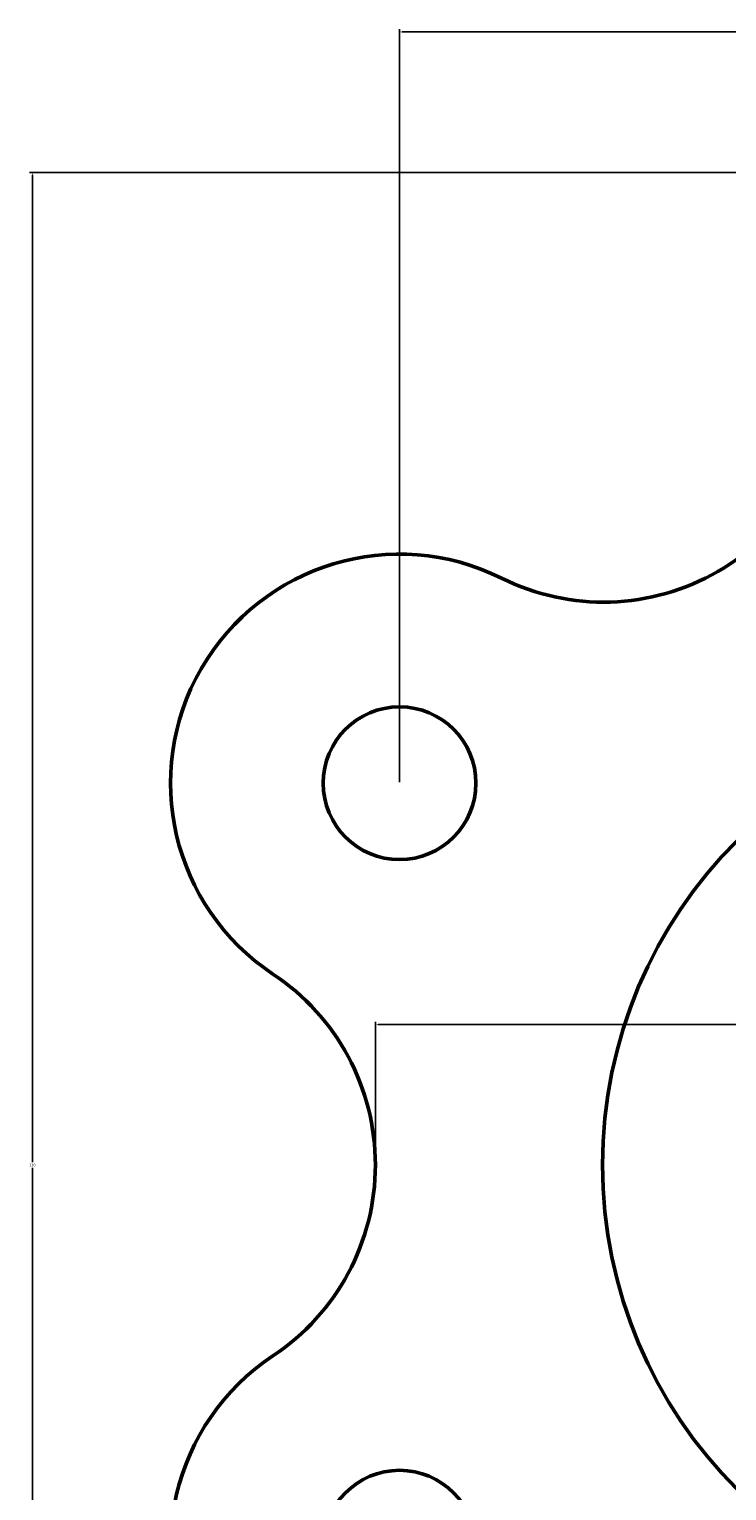
# Model space of a CAD drawing. Units: millimetres. Extents: x 2038 to 2173, y 1596 to 1745.
# Tile 2 of 4: x 2038 to 2084, y 1649 to 1745. Entities that reach past the tile are written whole.
import ezdxf

# ---------------------------------------------------------------- set-up
doc = ezdxf.new("R2010")
doc.units = ezdxf.units.MM
doc.layers.add('M-DIMS', color=2, linetype='Continuous', lineweight=18)
doc.layers.add('M-OUTL', color=7, linetype='Continuous', lineweight=50)
doc.styles.get("Standard").update_dxf_attribs({"font": 'arial.ttf'})
doc.dimstyles.get("Standard").update_dxf_attribs({"dimtxt": 0.18, "dimasz": 0.18, "dimexe": 0.18, "dimexo": 0.0625, "dimgap": 0.09, "dimtad": 0, "dimtih": 1, "dimtoh": 1, "dimdec": 4, "dimzin": 0, "dimdsep": 46, "dimtxsty": 'Standard', "dimcen": 0.09, "dimadec": 0, "dimazin": 0, "dimtfac": 1, "dimtdec": 4, "dimtofl": 0, "dimtmove": 0, "dimatfit": 3, "dimfxl": 1, "dimtolj": 1, "dimtzin": 0, "dimarcsym": 0})

# ---------------------------------------------------------------- blocks, each defined once
blk = doc.blocks.new('*U1')
blk.add_arc((-4.146, 7.965), 15, 243.55731, 356.44269)
blk = doc.blocks.new('*U2')
at = {"layer": 'M-OUTL', "color": 0, "linetype": 'ByBlock', "lineweight": -2, "transparency": 16777216}
blk.add_blockref('*U1', (2079.691, 1714.68), dxfattribs=at)
at = {"layer": 'M-OUTL', "color": 0, "linetype": 'ByBlock', "lineweight": -2, "transparency": 16777216, "rotation": 60.00000000000003}
blk.add_blockref('*U1', (2054.574, 1670.392), dxfattribs=at)
blk = doc.blocks.new('FLANGE-LUG-D10')
blk.add_circle((0, 0), 5)
blk.add_arc((0, 0), 15, 3.55731, 176.44269)
blk = doc.blocks.new('*D5')
at = {"layer": 'Defpoints', "color": 0, "transparency": 16777216}
for p in [(2038.131, 1735.784), (2105.488, 1735.784), (2105.488, 1605.784)]:
    blk.add_point(p, dxfattribs=at)
at = {"layer": 'M-DIMS', "color": 0, "lineweight": -2, "transparency": 16777216}
for p, q in [((2105.425, 1735.784), (2037.951, 1735.784)), ((2038.131, 1735.604), (2038.131, 1670.966)), ((2038.131, 1605.964), (2038.131, 1670.602)), ((2105.425, 1605.784), (2037.951, 1605.784))]:
    blk.add_line(p, q, dxfattribs=at)
at = {"layer": 'M-DIMS', "color": 0, "transparency": 16777216}
for points in [[(2038.101, 1735.604), (2038.161, 1735.604), (2038.131, 1735.784)], [(2038.101, 1605.964), (2038.161, 1605.964), (2038.131, 1605.784)]]:
    blk.add_solid(points, dxfattribs=at)
at = {"layer": 'M-DIMS', "color": 0, "transparency": 16777216, "insert": (2038.131, 1670.784), "char_height": 0.18, "attachment_point": 5}
blk.add_mtext('\\A1;130', dxfattribs=at)
blk = doc.blocks.new('*D8')
at = {"layer": 'Defpoints', "color": 0, "transparency": 16777216}
for p in [(2148.789, 1744.984), (2062.186, 1695.784), (2148.789, 1695.784)]:
    blk.add_point(p, dxfattribs=at)
at = {"layer": 'M-DIMS', "color": 0, "lineweight": -2, "transparency": 16777216}
for p, q in [((2062.186, 1695.847), (2062.186, 1745.164)), ((2062.366, 1744.984), (2105.164, 1744.984)), ((2148.609, 1744.984), (2105.812, 1744.984)), ((2148.789, 1695.847), (2148.789, 1745.164))]:
    blk.add_line(p, q, dxfattribs=at)
at = {"layer": 'M-DIMS', "color": 0, "transparency": 16777216}
for points in [[(2062.366, 1745.014), (2062.366, 1744.954), (2062.186, 1744.984)], [(2148.609, 1745.014), (2148.609, 1744.954), (2148.789, 1744.984)]]:
    blk.add_solid(points, dxfattribs=at)
at = {"layer": 'M-DIMS', "color": 0, "transparency": 16777216, "insert": (2105.488, 1744.984), "char_height": 0.18, "attachment_point": 5}
blk.add_mtext('\\A1;86.6', dxfattribs=at)
blk = doc.blocks.new('*D9')
at = {"layer": 'Defpoints', "color": 0, "transparency": 16777216}
for p in [(2150.372, 1679.984), (2060.603, 1670.784), (2150.372, 1670.784)]:
    blk.add_point(p, dxfattribs=at)
at = {"layer": 'M-DIMS', "color": 0, "lineweight": -2, "transparency": 16777216}
for p, q in [((2060.603, 1670.847), (2060.603, 1680.164)), ((2060.783, 1679.984), (2105.094, 1679.984)), ((2150.192, 1679.984), (2105.882, 1679.984)), ((2150.372, 1670.847), (2150.372, 1680.164))]:
    blk.add_line(p, q, dxfattribs=at)
at = {"layer": 'M-DIMS', "color": 0, "transparency": 16777216}
for points in [[(2060.783, 1680.014), (2060.783, 1679.954), (2060.603, 1679.984)], [(2150.192, 1680.014), (2150.192, 1679.954), (2150.372, 1679.984)]]:
    blk.add_solid(points, dxfattribs=at)
at = {"layer": 'M-DIMS', "color": 0, "transparency": 16777216, "insert": (2105.488, 1679.984), "char_height": 0.18, "attachment_point": 5}
blk.add_mtext('\\A1;89.77', dxfattribs=at)

msp = doc.modelspace()

# ---------------------------------------------------------------- linework, layer by layer
at = {"layer": 'M-OUTL'}
msp.add_circle((2105.488, 1670.784), 30, dxfattribs=at)

# ---------------------------------------------------------------- block references
msp.add_blockref('*U2', (0, 0), dxfattribs=at)
for p, rotation in [((2062.186, 1695.784), 60.00000000000067), ((2062.186, 1645.784), 120.0000000000013)]:
    msp.add_blockref('FLANGE-LUG-D10', p, dxfattribs=dict(at, rotation=rotation))

# ---------------------------------------------------------------- dimensions: what is measured, and where the dimension line sits
at = {"layer": 'M-DIMS'}
for base, p1, p2, override, picture, middle in [((2148.789, 1744.984), (2062.186, 1695.784), (2148.789, 1695.784), {"dimdec": 1, "dimlfac": 1, "dimrnd": 0, "dimzin": 0, "dimdsep": 46, "dimlunit": 2}, '*D8', (2105.488, 1744.984)), ((2150.372, 1679.984), (2060.603, 1670.784), (2150.372, 1670.784), {"dimdec": 2, "dimlfac": 1, "dimrnd": 0, "dimzin": 0, "dimdsep": 46, "dimlunit": 2}, '*D9', (2105.488, 1679.984))]:
    dim = msp.add_linear_dim(base=base, p1=p1, p2=p2, dimstyle='Standard', override=override, dxfattribs=at)
    dim.commit()
    dim.dimension.update_dxf_attribs({"geometry": picture, "text_midpoint": middle})
dim = msp.add_linear_dim(base=(2038.131, 1735.784), p1=(2105.488, 1605.784), p2=(2105.488, 1735.784), angle=90, dimstyle='Standard', override={"dimdec": 0, "dimlfac": 1, "dimrnd": 0, "dimzin": 0, "dimdsep": 46, "dimlunit": 2}, dxfattribs=at)
dim.commit()
dim.dimension.update_dxf_attribs({"geometry": '*D5', "text_midpoint": (2038.131, 1670.784)})

doc.saveas('drawing.dxf')
